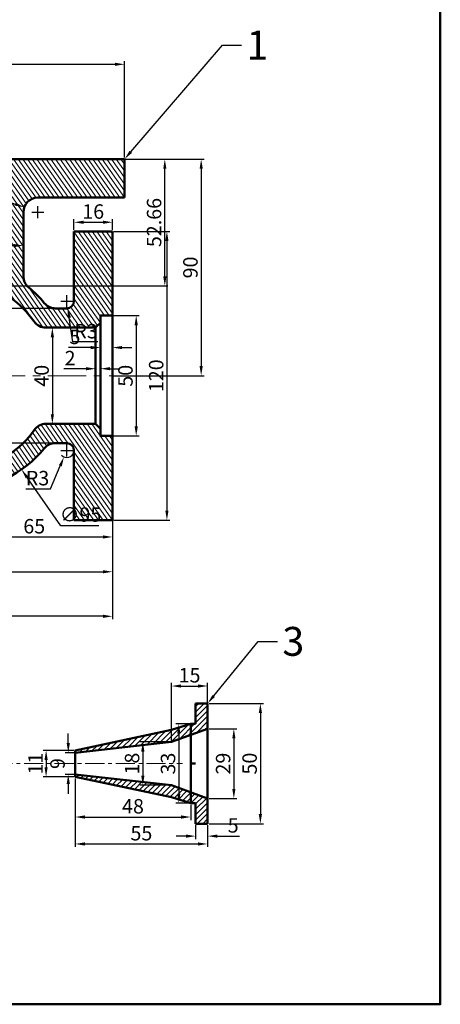
# Model space of a CAD drawing. Units: millimetres. Extents: x 39 to 520, y -165 to 464.
# Tile 3 of 4: x 345 to 520, y -165 to 244. Entities that reach past the tile are written whole.
import ezdxf
from ezdxf import colors
from ezdxf.entities.mleader import LeaderData, LeaderLine
from ezdxf.math import Vec2, Vec3

# ---------------------------------------------------------------- set-up
doc = ezdxf.new("R2010")
doc.units = ezdxf.units.MM
doc.header["$LTSCALE"] = 0.5
doc.linetypes.add('CENTER', pattern=[50.8, 31.75, -6.35, 6.35, -6.35])
for name, color, linetype, lineweight in [('M-CNTR', 1, 'CENTER', 18), ('M-DIMS', 2, 'Continuous', 25), ('M-HATC', 8, 'Continuous', 18), ('M-OUTL', 7, 'Continuous', 50), ('M-TEXT', 3, 'Continuous', 25), ('M-TTLB', 7, 'Continuous', 50)]:
    doc.layers.add(name, color=color, linetype=linetype, lineweight=lineweight)
doc.styles.get("Standard").update_dxf_attribs({"font": 'arial.ttf'})
doc.dimstyles.new('ISO-25', dxfattribs={"dimtxt": 6, "dimasz": 4, "dimexe": 1.25, "dimexo": 0.625, "dimtad": 1, "dimtoh": 1, "dimdec": 1, "dimtxsty": 'Standard', "dimcen": 2.5, "dimadec": 0, "dimazin": 0, "dimtfac": 1, "dimtdec": 1, "dimtofl": 0, "dimtmove": 0, "dimatfit": 3, "dimfxl": 1, "dimarcsym": 0})

# ---------------------------------------------------------------- blocks, each defined once
blk = doc.blocks.new('*D1')
at = {"layer": 'Defpoints', "color": 0, "ltscale": 0.5, "transparency": 16777216}
for p in [(388.62, 225.52), (248.62, 186.1), (388.62, 186.1)]:
    blk.add_point(p, dxfattribs=at)
at = {"layer": 'M-DIMS', "color": 0, "lineweight": -2, "ltscale": 0.5, "transparency": 16777216}
for p, q in [((248.62, 186.73), (248.62, 226.77)), ((252.62, 225.52), (384.62, 225.52)), ((388.62, 186.73), (388.62, 226.77))]:
    blk.add_line(p, q, dxfattribs=at)
at = {"layer": 'M-DIMS', "color": 0, "ltscale": 0.5, "transparency": 16777216}
for points in [[(252.62, 226.18), (252.62, 224.85), (248.62, 225.52)], [(384.62, 226.18), (384.62, 224.85), (388.62, 225.52)]]:
    blk.add_solid(points, dxfattribs=at)
at = {"layer": 'M-DIMS', "color": 0, "ltscale": 0.5, "transparency": 16777216, "insert": (318.62, 229.21), "char_height": 6, "attachment_point": 5}
blk.add_mtext('140', dxfattribs=at)
blk = doc.blocks.new('*D2')
at = {"layer": 'Defpoints', "color": 0, "ltscale": 0.5, "transparency": 16777216}
for p in [(290.62, 156.95), (346.62, 156.95), (346.62, 150.19)]:
    blk.add_point(p, dxfattribs=at)
at = {"layer": 'M-DIMS', "color": 0, "lineweight": -2, "ltscale": 0.5, "transparency": 16777216}
for p, q in [((290.62, 156.32), (290.62, 148.94)), ((346.62, 156.32), (346.62, 148.94)), ((294.62, 150.19), (342.62, 150.19))]:
    blk.add_line(p, q, dxfattribs=at)
at = {"layer": 'M-DIMS', "color": 0, "ltscale": 0.5, "transparency": 16777216}
for points in [[(294.62, 150.85), (294.62, 149.52), (290.62, 150.19)], [(342.62, 150.85), (342.62, 149.52), (346.62, 150.19)]]:
    blk.add_solid(points, dxfattribs=at)
at = {"layer": 'M-DIMS', "color": 0, "ltscale": 0.5, "transparency": 16777216, "insert": (318.62, 153.88), "char_height": 6, "attachment_point": 5}
blk.add_mtext('56', dxfattribs=at)
blk = doc.blocks.new('*D4')
at = {"layer": 'Defpoints', "color": 0, "ltscale": 0.5, "transparency": 16777216}
for p in [(383.62, 159.88), (367.62, 156.1), (383.62, 156.1)]:
    blk.add_point(p, dxfattribs=at)
at = {"layer": 'M-DIMS', "color": 0, "lineweight": -2, "ltscale": 0.5, "transparency": 16777216}
for p, q in [((367.62, 156.73), (367.62, 161.13)), ((371.62, 159.88), (379.62, 159.88)), ((383.62, 156.73), (383.62, 161.13))]:
    blk.add_line(p, q, dxfattribs=at)
at = {"layer": 'M-DIMS', "color": 0, "ltscale": 0.5, "transparency": 16777216}
for points in [[(371.62, 160.55), (371.62, 159.22), (367.62, 159.88)], [(379.62, 160.55), (379.62, 159.22), (383.62, 159.88)]]:
    blk.add_solid(points, dxfattribs=at)
at = {"layer": 'M-DIMS', "color": 0, "ltscale": 0.5, "transparency": 16777216, "insert": (375.62, 163.57), "char_height": 6, "attachment_point": 5}
blk.add_mtext('16', dxfattribs=at)
blk = doc.blocks.new('*D6')
at = {"layer": 'Defpoints', "color": 0, "ltscale": 0.5, "transparency": 16777216}
for p in [(388.62, 186.1), (383.62, 96.1), (420.47, 96.1)]:
    blk.add_point(p, dxfattribs=at)
at = {"layer": 'M-DIMS', "color": 0, "lineweight": -2, "ltscale": 0.5, "transparency": 16777216}
for p, q in [((389.25, 186.1), (421.72, 186.1)), ((420.47, 182.1), (420.47, 100.1)), ((384.25, 96.1), (421.72, 96.1))]:
    blk.add_line(p, q, dxfattribs=at)
at = {"layer": 'M-DIMS', "color": 0, "ltscale": 0.5, "transparency": 16777216}
for points in [[(419.81, 182.1), (421.14, 182.1), (420.47, 186.1)], [(419.81, 100.1), (421.14, 100.1), (420.47, 96.1)]]:
    blk.add_solid(points, dxfattribs=at)
at = {"layer": 'M-DIMS', "color": 0, "ltscale": 0.5, "transparency": 16777216, "insert": (416.78, 141.1), "char_height": 6, "attachment_point": 5, "rotation": 90}
blk.add_mtext('90', dxfattribs=at)
blk = doc.blocks.new('*D7')
at = {"layer": 'Defpoints', "color": 0, "ltscale": 0.5, "transparency": 16777216}
for p in [(383.62, 156.1), (383.62, 36.1), (406.24, 36.1)]:
    blk.add_point(p, dxfattribs=at)
at = {"layer": 'M-DIMS', "color": 0, "lineweight": -2, "ltscale": 0.5, "transparency": 16777216}
for p, q in [((384.25, 156.1), (407.49, 156.1)), ((406.24, 152.1), (406.24, 40.1)), ((384.25, 36.1), (407.49, 36.1))]:
    blk.add_line(p, q, dxfattribs=at)
at = {"layer": 'M-DIMS', "color": 0, "ltscale": 0.5, "transparency": 16777216}
for points in [[(405.57, 152.1), (406.9, 152.1), (406.24, 156.1)], [(405.57, 40.1), (406.9, 40.1), (406.24, 36.1)]]:
    blk.add_solid(points, dxfattribs=at)
at = {"layer": 'M-DIMS', "color": 0, "ltscale": 0.5, "transparency": 16777216, "insert": (402.55, 96.1), "char_height": 6, "attachment_point": 5, "rotation": 90}
blk.add_mtext('120', dxfattribs=at)
blk = doc.blocks.new('*D8')
at = {"layer": 'Defpoints', "color": 0, "ltscale": 0.5, "transparency": 16777216}
for p in [(383.62, 121.1), (383.62, 71.1), (393.48, 71.1)]:
    blk.add_point(p, dxfattribs=at)
at = {"layer": 'M-DIMS', "color": 0, "lineweight": -2, "ltscale": 0.5, "transparency": 16777216}
for p, q in [((384.25, 121.1), (394.73, 121.1)), ((393.48, 117.1), (393.48, 75.1)), ((384.25, 71.1), (394.73, 71.1))]:
    blk.add_line(p, q, dxfattribs=at)
at = {"layer": 'M-DIMS', "color": 0, "ltscale": 0.5, "transparency": 16777216}
for points in [[(392.81, 117.1), (394.15, 117.1), (393.48, 121.1)], [(392.81, 75.1), (394.15, 75.1), (393.48, 71.1)]]:
    blk.add_solid(points, dxfattribs=at)
at = {"layer": 'M-DIMS', "color": 0, "ltscale": 0.5, "transparency": 16777216, "insert": (389.79, 96.1), "char_height": 6, "attachment_point": 5, "rotation": 90}
blk.add_mtext('50', dxfattribs=at)
blk = doc.blocks.new('*D9')
at = {"layer": 'Defpoints', "color": 0, "ltscale": 0.5, "transparency": 16777216}
for p in [(378.62, 106.38), (383.62, 107.8), (383.62, 106.38)]:
    blk.add_point(p, dxfattribs=at)
at = {"layer": 'M-DIMS', "color": 0, "lineweight": -2, "ltscale": 0.5, "transparency": 16777216}
for p, q in [((374.62, 107.8), (365.39, 107.8)), ((378.62, 107.01), (378.62, 109.05)), ((383.62, 107.01), (383.62, 109.05)), ((387.62, 107.8), (391.62, 107.8))]:
    blk.add_line(p, q, dxfattribs=at)
at = {"layer": 'M-DIMS', "color": 0, "ltscale": 0.5, "transparency": 16777216}
for points in [[(374.62, 108.47), (374.62, 107.13), (378.62, 107.8)], [(387.62, 108.47), (387.62, 107.13), (383.62, 107.8)]]:
    blk.add_solid(points, dxfattribs=at)
at = {"layer": 'M-DIMS', "color": 0, "ltscale": 0.5, "transparency": 16777216, "insert": (368.01, 111.47), "char_height": 6, "attachment_point": 5}
blk.add_mtext('5', dxfattribs=at)
blk = doc.blocks.new('*D10')
at = {"layer": 'Defpoints', "color": 0, "ltscale": 0.5, "transparency": 16777216}
for p in [(376.62, 99.43), (378.62, 99.43), (378.62, 99.03)]:
    blk.add_point(p, dxfattribs=at)
at = {"layer": 'M-DIMS', "color": 0, "lineweight": -2, "ltscale": 0.5, "transparency": 16777216}
for p, q in [((372.62, 99.03), (363.4, 99.03)), ((376.62, 98.8), (376.62, 97.78)), ((378.62, 98.8), (378.62, 97.78)), ((382.62, 99.03), (386.62, 99.03))]:
    blk.add_line(p, q, dxfattribs=at)
at = {"layer": 'M-DIMS', "color": 0, "ltscale": 0.5, "transparency": 16777216}
for points in [[(372.62, 99.69), (372.62, 98.36), (376.62, 99.03)], [(382.62, 99.69), (382.62, 98.36), (378.62, 99.03)]]:
    blk.add_solid(points, dxfattribs=at)
at = {"layer": 'M-DIMS', "color": 0, "ltscale": 0.5, "transparency": 16777216, "insert": (366.01, 102.66), "char_height": 6, "attachment_point": 5}
blk.add_mtext('2', dxfattribs=at)
blk = doc.blocks.new('*D11')
at = {"layer": 'Defpoints', "color": 0, "ltscale": 0.5, "transparency": 16777216}
for p in [(318.62, 41.45), (383.62, 36.1), (383.62, 29.1)]:
    blk.add_point(p, dxfattribs=at)
at = {"layer": 'M-DIMS', "color": 0, "lineweight": -2, "ltscale": 0.5, "transparency": 16777216}
for p, q in [((318.62, 40.83), (318.62, 27.85)), ((383.62, 35.48), (383.62, 27.85)), ((322.62, 29.1), (379.62, 29.1))]:
    blk.add_line(p, q, dxfattribs=at)
at = {"layer": 'M-DIMS', "color": 0, "ltscale": 0.5, "transparency": 16777216}
for points in [[(322.62, 29.77), (322.62, 28.44), (318.62, 29.1)], [(379.62, 29.77), (379.62, 28.44), (383.62, 29.1)]]:
    blk.add_solid(points, dxfattribs=at)
at = {"layer": 'M-DIMS', "color": 0, "ltscale": 0.5, "transparency": 16777216, "insert": (351.12, 32.79), "char_height": 6, "attachment_point": 5}
blk.add_mtext('65', dxfattribs=at)
blk = doc.blocks.new('*D12')
at = {"layer": 'Defpoints', "color": 0, "ltscale": 0.5, "transparency": 16777216}
for p in [(283.62, 96.1), (383.62, 48.96), (383.62, 14.65)]:
    blk.add_point(p, dxfattribs=at)
at = {"layer": 'M-DIMS', "color": 0, "lineweight": -2, "ltscale": 0.5, "transparency": 16777216}
for p, q in [((283.62, 95.48), (283.62, 13.4)), ((383.62, 48.34), (383.62, 13.4)), ((287.62, 14.65), (379.62, 14.65))]:
    blk.add_line(p, q, dxfattribs=at)
at = {"layer": 'M-DIMS', "color": 0, "ltscale": 0.5, "transparency": 16777216}
for points in [[(287.62, 15.32), (287.62, 13.98), (283.62, 14.65)], [(379.62, 15.32), (379.62, 13.98), (383.62, 14.65)]]:
    blk.add_solid(points, dxfattribs=at)
at = {"layer": 'M-DIMS', "color": 0, "ltscale": 0.5, "transparency": 16777216, "insert": (333.62, 18.34), "char_height": 6, "attachment_point": 5}
blk.add_mtext('100', dxfattribs=at)
blk = doc.blocks.new('*D13')
at = {"layer": 'Defpoints', "color": 0, "ltscale": 0.5, "transparency": 16777216}
for p in [(153.62, 36.1), (383.62, 36.1), (153.62, -3.86)]:
    blk.add_point(p, dxfattribs=at)
at = {"layer": 'M-DIMS', "color": 0, "lineweight": -2, "ltscale": 0.5, "transparency": 16777216}
for p, q in [((153.62, 35.48), (153.62, -5.11)), ((383.62, 35.48), (383.62, -5.11)), ((379.62, -3.86), (157.62, -3.86))]:
    blk.add_line(p, q, dxfattribs=at)
at = {"layer": 'M-DIMS', "color": 0, "ltscale": 0.5, "transparency": 16777216}
for points in [[(157.62, -3.19), (157.62, -4.53), (153.62, -3.86)], [(379.62, -3.19), (379.62, -4.53), (383.62, -3.86)]]:
    blk.add_solid(points, dxfattribs=at)
at = {"layer": 'M-DIMS', "color": 0, "ltscale": 0.5, "transparency": 16777216, "insert": (268.62, -0.17), "char_height": 6, "attachment_point": 5}
blk.add_mtext('230', dxfattribs=at)
blk = doc.blocks.new('*D14')
at = {"layer": 'Defpoints', "color": 0, "ltscale": 0.5, "transparency": 16777216}
for p in [(359.93, 124.1), (340.68, 68.1), (362.28, 68.1)]:
    blk.add_point(p, dxfattribs=at)
at = {"layer": 'M-DIMS', "color": 0, "lineweight": -2, "ltscale": 0.5, "transparency": 16777216}
for p, q in [((359.3, 124.1), (339.43, 124.1)), ((340.68, 120.1), (340.68, 72.1)), ((361.65, 68.1), (339.43, 68.1))]:
    blk.add_line(p, q, dxfattribs=at)
at = {"layer": 'M-DIMS', "color": 0, "ltscale": 0.5, "transparency": 16777216}
for points in [[(340.02, 120.1), (341.35, 120.1), (340.68, 124.1)], [(340.02, 72.1), (341.35, 72.1), (340.68, 68.1)]]:
    blk.add_solid(points, dxfattribs=at)
at = {"layer": 'M-DIMS', "color": 0, "ltscale": 0.5, "transparency": 16777216, "insert": (337, 96.1), "char_height": 6, "attachment_point": 5, "rotation": 90}
blk.add_mtext('56', dxfattribs=at)
blk = doc.blocks.new('*D15')
at = {"layer": 'Defpoints', "color": 0, "ltscale": 0.5, "transparency": 16777216}
for p in [(361.76, 116.1), (358.64, 76.1), (361.76, 76.1)]:
    blk.add_point(p, dxfattribs=at)
at = {"layer": 'M-DIMS', "color": 0, "lineweight": -2, "ltscale": 0.5, "transparency": 16777216}
for p, q in [((361.13, 116.1), (357.39, 116.1)), ((358.64, 112.1), (358.64, 80.1)), ((361.13, 76.1), (357.39, 76.1))]:
    blk.add_line(p, q, dxfattribs=at)
at = {"layer": 'M-DIMS', "color": 0, "ltscale": 0.5, "transparency": 16777216}
for points in [[(357.98, 112.1), (359.31, 112.1), (358.64, 116.1)], [(357.98, 80.1), (359.31, 80.1), (358.64, 76.1)]]:
    blk.add_solid(points, dxfattribs=at)
at = {"layer": 'M-DIMS', "color": 0, "ltscale": 0.5, "transparency": 16777216, "insert": (354.95, 96.1), "char_height": 6, "attachment_point": 5, "rotation": 90}
blk.add_mtext('40', dxfattribs=at)
blk = doc.blocks.new('*D30')
at = {"layer": 'Defpoints', "color": 0, "ltscale": 0.5, "transparency": 16777216}
for p in [(363.47, 62.33), (364.62, 65.1)]:
    blk.add_point(p, dxfattribs=at)
at = {"layer": 'M-DIMS', "color": 0, "lineweight": -2, "ltscale": 0.5, "transparency": 16777216}
for p, q in [((364.62, 62.6), (364.62, 67.6)), ((362.12, 65.1), (367.12, 65.1)), ((357.94, 49.09), (361.93, 58.64)), ((347.64, 49.09), (357.94, 49.09))]:
    blk.add_line(p, q, dxfattribs=at)
blk.add_arc((364.62, 65.1), 3, 223.4691, 348.0634, dxfattribs=at)
at = {"layer": 'M-DIMS', "color": 0, "ltscale": 0.5, "transparency": 16777216}
blk.add_solid([(361.31, 58.9), (362.54, 58.39), (363.47, 62.33)], dxfattribs=at)
at = {"layer": 'M-DIMS', "color": 0, "ltscale": 0.5, "transparency": 16777216, "insert": (352.48, 52.78), "char_height": 6, "attachment_point": 5}
blk.add_mtext('R3', dxfattribs=at)
blk = doc.blocks.new('*D48')
at = {"layer": 'Defpoints', "color": 0, "ltscale": 0.5, "transparency": 16777216}
for p in [(423.14, -32.82), (408.14, -56.06), (423.14, -56.06)]:
    blk.add_point(p, dxfattribs=at)
at = {"layer": 'M-DIMS', "color": 0, "lineweight": -2, "ltscale": 0.5, "transparency": 16777216}
for p, q in [((408.14, -55.44), (408.14, -31.57)), ((423.14, -55.44), (423.14, -31.57)), ((412.14, -32.82), (419.14, -32.82))]:
    blk.add_line(p, q, dxfattribs=at)
at = {"layer": 'M-DIMS', "color": 0, "ltscale": 0.5, "transparency": 16777216}
for points in [[(412.14, -32.16), (412.14, -33.49), (408.14, -32.82)], [(419.14, -32.16), (419.14, -33.49), (423.14, -32.82)]]:
    blk.add_solid(points, dxfattribs=at)
at = {"layer": 'M-DIMS', "color": 0, "ltscale": 0.5, "transparency": 16777216, "insert": (415.64, -29.14), "char_height": 6, "attachment_point": 5}
blk.add_mtext('15', dxfattribs=at)
blk = doc.blocks.new('*D49')
at = {"layer": 'Defpoints', "color": 0, "ltscale": 0.5, "transparency": 16777216}
for p in [(423.14, -50.56), (423.14, -79.56), (434.05, -79.56)]:
    blk.add_point(p, dxfattribs=at)
at = {"layer": 'M-DIMS', "color": 0, "lineweight": -2, "ltscale": 0.5, "transparency": 16777216}
for p, q in [((423.77, -50.56), (435.3, -50.56)), ((434.05, -54.56), (434.05, -75.56)), ((423.77, -79.56), (435.3, -79.56))]:
    blk.add_line(p, q, dxfattribs=at)
at = {"layer": 'M-DIMS', "color": 0, "ltscale": 0.5, "transparency": 16777216}
for points in [[(433.39, -54.56), (434.72, -54.56), (434.05, -50.56)], [(433.39, -75.56), (434.72, -75.56), (434.05, -79.56)]]:
    blk.add_solid(points, dxfattribs=at)
at = {"layer": 'M-DIMS', "color": 0, "ltscale": 0.5, "transparency": 16777216, "insert": (430.37, -65.06), "char_height": 6, "attachment_point": 5, "rotation": 90}
blk.add_mtext('29', dxfattribs=at)
blk = doc.blocks.new('*D50')
at = {"layer": 'Defpoints', "color": 0, "ltscale": 0.5, "transparency": 16777216}
for p in [(423.14, -40.06), (423.14, -90.06), (445.07, -90.06)]:
    blk.add_point(p, dxfattribs=at)
at = {"layer": 'M-DIMS', "color": 0, "lineweight": -2, "ltscale": 0.5, "transparency": 16777216}
for p, q in [((423.77, -40.06), (446.32, -40.06)), ((445.07, -44.06), (445.07, -86.06)), ((423.77, -90.06), (446.32, -90.06))]:
    blk.add_line(p, q, dxfattribs=at)
at = {"layer": 'M-DIMS', "color": 0, "ltscale": 0.5, "transparency": 16777216}
for points in [[(444.4, -44.06), (445.74, -44.06), (445.07, -40.06)], [(444.4, -86.06), (445.74, -86.06), (445.07, -90.06)]]:
    blk.add_solid(points, dxfattribs=at)
at = {"layer": 'M-DIMS', "color": 0, "ltscale": 0.5, "transparency": 16777216, "insert": (441.38, -65.06), "char_height": 6, "attachment_point": 5, "rotation": 90}
blk.add_mtext('50', dxfattribs=at)
blk = doc.blocks.new('*D51')
at = {"layer": 'Defpoints', "color": 0, "ltscale": 0.5, "transparency": 16777216}
for p in [(368.14, -70.56), (423.14, -90.06), (423.14, -98.46)]:
    blk.add_point(p, dxfattribs=at)
at = {"layer": 'M-DIMS', "color": 0, "lineweight": -2, "ltscale": 0.5, "transparency": 16777216}
for p, q in [((368.14, -71.19), (368.14, -99.71)), ((423.14, -90.69), (423.14, -99.71)), ((372.14, -98.46), (419.14, -98.46))]:
    blk.add_line(p, q, dxfattribs=at)
at = {"layer": 'M-DIMS', "color": 0, "ltscale": 0.5, "transparency": 16777216}
for points in [[(372.14, -97.79), (372.14, -99.12), (368.14, -98.46)], [(419.14, -97.79), (419.14, -99.12), (423.14, -98.46)]]:
    blk.add_solid(points, dxfattribs=at)
at = {"layer": 'M-DIMS', "color": 0, "ltscale": 0.5, "transparency": 16777216, "insert": (395.64, -94.78), "char_height": 6, "attachment_point": 5}
blk.add_mtext('55', dxfattribs=at)
blk = doc.blocks.new('*D52')
at = {"layer": 'Defpoints', "color": 0, "ltscale": 0.5, "transparency": 16777216}
for p in [(368.14, -76.99), (416.14, -81.56), (416.14, -87.26)]:
    blk.add_point(p, dxfattribs=at)
at = {"layer": 'M-DIMS', "color": 0, "lineweight": -2, "ltscale": 0.5, "transparency": 16777216}
for p, q in [((368.14, -77.62), (368.14, -88.51)), ((416.14, -82.19), (416.14, -88.51)), ((372.14, -87.26), (412.14, -87.26))]:
    blk.add_line(p, q, dxfattribs=at)
at = {"layer": 'M-DIMS', "color": 0, "ltscale": 0.5, "transparency": 16777216}
for points in [[(372.14, -86.59), (372.14, -87.93), (368.14, -87.26)], [(412.14, -86.59), (412.14, -87.93), (416.14, -87.26)]]:
    blk.add_solid(points, dxfattribs=at)
at = {"layer": 'M-DIMS', "color": 0, "ltscale": 0.5, "transparency": 16777216, "insert": (392.14, -83.57), "char_height": 6, "attachment_point": 5}
blk.add_mtext('48', dxfattribs=at)
blk = doc.blocks.new('*D53')
at = {"layer": 'Defpoints', "color": 0, "ltscale": 0.5, "transparency": 16777216}
for p in [(368.14, -60.56), (365.25, -69.56), (368.14, -69.56)]:
    blk.add_point(p, dxfattribs=at)
at = {"layer": 'M-DIMS', "color": 0, "lineweight": -2, "ltscale": 0.5, "transparency": 16777216}
for p, q in [((365.25, -56.56), (365.25, -52.56)), ((367.52, -60.56), (364, -60.56)), ((367.52, -69.56), (364, -69.56)), ((365.25, -73.56), (365.25, -77.56))]:
    blk.add_line(p, q, dxfattribs=at)
at = {"layer": 'M-DIMS', "color": 0, "ltscale": 0.5, "transparency": 16777216}
for points in [[(364.59, -56.56), (365.92, -56.56), (365.25, -60.56)], [(364.59, -73.56), (365.92, -73.56), (365.25, -69.56)]]:
    blk.add_solid(points, dxfattribs=at)
at = {"layer": 'M-DIMS', "color": 0, "ltscale": 0.5, "transparency": 16777216, "insert": (361.56, -65.06), "char_height": 6, "attachment_point": 5, "rotation": 90}
blk.add_mtext('9', dxfattribs=at)
blk = doc.blocks.new('*D54')
at = {"layer": 'Defpoints', "color": 0, "ltscale": 0.5, "transparency": 16777216}
for p in [(368.14, -59.56), (356.04, -70.56), (368.14, -70.56)]:
    blk.add_point(p, dxfattribs=at)
at = {"layer": 'M-DIMS', "color": 0, "lineweight": -2, "ltscale": 0.5, "transparency": 16777216}
for p, q in [((367.52, -59.56), (354.79, -59.56)), ((356.04, -63.56), (356.04, -66.56)), ((367.52, -70.56), (354.79, -70.56))]:
    blk.add_line(p, q, dxfattribs=at)
at = {"layer": 'M-DIMS', "color": 0, "ltscale": 0.5, "transparency": 16777216}
for points in [[(355.37, -63.56), (356.71, -63.56), (356.04, -59.56)], [(355.37, -66.56), (356.71, -66.56), (356.04, -70.56)]]:
    blk.add_solid(points, dxfattribs=at)
at = {"layer": 'M-DIMS', "color": 0, "ltscale": 0.5, "transparency": 16777216, "insert": (352.4, -65.06), "char_height": 6, "attachment_point": 5, "rotation": 90}
blk.add_mtext('11', dxfattribs=at)
blk = doc.blocks.new('*D55')
at = {"layer": 'Defpoints', "color": 0, "ltscale": 0.5, "transparency": 16777216}
for p in [(418.14, -48.56), (411.17, -81.56), (418.14, -81.56)]:
    blk.add_point(p, dxfattribs=at)
at = {"layer": 'M-DIMS', "color": 0, "lineweight": -2, "ltscale": 0.5, "transparency": 16777216}
for p, q in [((417.52, -48.56), (409.92, -48.56)), ((411.17, -52.56), (411.17, -77.56)), ((417.52, -81.56), (409.92, -81.56))]:
    blk.add_line(p, q, dxfattribs=at)
at = {"layer": 'M-DIMS', "color": 0, "ltscale": 0.5, "transparency": 16777216}
for points in [[(410.51, -52.56), (411.84, -52.56), (411.17, -48.56)], [(410.51, -77.56), (411.84, -77.56), (411.17, -81.56)]]:
    blk.add_solid(points, dxfattribs=at)
at = {"layer": 'M-DIMS', "color": 0, "ltscale": 0.5, "transparency": 16777216, "insert": (407.48, -65.06), "char_height": 6, "attachment_point": 5, "rotation": 90}
blk.add_mtext('33', dxfattribs=at)
blk = doc.blocks.new('*D56')
at = {"layer": 'Defpoints', "color": 0, "ltscale": 0.5, "transparency": 16777216}
for p in [(408.14, -56.06), (396.23, -74.06), (408.14, -74.06)]:
    blk.add_point(p, dxfattribs=at)
at = {"layer": 'M-DIMS', "color": 0, "lineweight": -2, "ltscale": 0.5, "transparency": 16777216}
for p, q in [((407.52, -56.06), (394.98, -56.06)), ((396.23, -60.06), (396.23, -70.06)), ((407.52, -74.06), (394.98, -74.06))]:
    blk.add_line(p, q, dxfattribs=at)
at = {"layer": 'M-DIMS', "color": 0, "ltscale": 0.5, "transparency": 16777216}
for points in [[(395.56, -60.06), (396.9, -60.06), (396.23, -56.06)], [(395.56, -70.06), (396.9, -70.06), (396.23, -74.06)]]:
    blk.add_solid(points, dxfattribs=at)
at = {"layer": 'M-DIMS', "color": 0, "ltscale": 0.5, "transparency": 16777216, "insert": (392.54, -65.06), "char_height": 6, "attachment_point": 5, "rotation": 90}
blk.add_mtext('18', dxfattribs=at)
blk = doc.blocks.new('*D57')
at = {"layer": 'Defpoints', "color": 0, "ltscale": 0.5, "transparency": 16777216}
for p in [(418.14, -90.06), (423.14, -90.06), (423.14, -95.2)]:
    blk.add_point(p, dxfattribs=at)
at = {"layer": 'M-DIMS', "color": 0, "lineweight": -2, "ltscale": 0.5, "transparency": 16777216}
for p, q in [((418.14, -90.69), (418.14, -96.45)), ((423.14, -90.69), (423.14, -96.45)), ((414.14, -95.2), (410.14, -95.2)), ((427.14, -95.2), (436.37, -95.2))]:
    blk.add_line(p, q, dxfattribs=at)
at = {"layer": 'M-DIMS', "color": 0, "ltscale": 0.5, "transparency": 16777216}
for points in [[(414.14, -94.53), (414.14, -95.86), (418.14, -95.2)], [(427.14, -94.53), (427.14, -95.86), (423.14, -95.2)]]:
    blk.add_solid(points, dxfattribs=at)
at = {"layer": 'M-DIMS', "color": 0, "ltscale": 0.5, "transparency": 16777216, "insert": (433.76, -91.52), "char_height": 6, "attachment_point": 5}
blk.add_mtext('5', dxfattribs=at)
blk = doc.blocks.new('*D58')
at = {"layer": 'Defpoints', "color": 0, "ltscale": 0.5, "transparency": 16777216}
for p in [(338.62, 186.1), (405.37, 186.1), (338.62, 133.44)]:
    blk.add_point(p, dxfattribs=at)
at = {"layer": 'M-DIMS', "color": 0, "lineweight": -2, "ltscale": 0.5, "transparency": 16777216}
for p, q in [((339.25, 186.1), (406.62, 186.1)), ((405.37, 137.44), (405.37, 182.1)), ((339.25, 133.44), (406.62, 133.44))]:
    blk.add_line(p, q, dxfattribs=at)
at = {"layer": 'M-DIMS', "color": 0, "ltscale": 0.5, "transparency": 16777216}
for points in [[(404.71, 182.1), (406.04, 182.1), (405.37, 186.1)], [(404.71, 137.44), (406.04, 137.44), (405.37, 133.44)]]:
    blk.add_solid(points, dxfattribs=at)
at = {"layer": 'M-DIMS', "color": 0, "ltscale": 0.5, "transparency": 16777216, "insert": (401.68, 159.77), "char_height": 6, "attachment_point": 5, "rotation": 90}
blk.add_mtext('52.66', dxfattribs=at)
blk = doc.blocks.new('*D62')
at = {"layer": 'Defpoints', "color": 0, "ltscale": 0.5, "transparency": 16777216}
for p in [(364.62, 127.1), (365.07, 124.14)]:
    blk.add_point(p, dxfattribs=at)
at = {"layer": 'M-DIMS', "color": 0, "lineweight": -2, "ltscale": 0.5, "transparency": 16777216}
for p, q in [((362.12, 127.1), (367.12, 127.1)), ((364.62, 124.6), (364.62, 129.6)), ((367.18, 110.16), (365.67, 120.18)), ((377.48, 110.16), (367.18, 110.16))]:
    blk.add_line(p, q, dxfattribs=at)
at = {"layer": 'M-DIMS', "color": 0, "ltscale": 0.5, "transparency": 16777216}
blk.add_solid([(366.33, 120.28), (365.01, 120.08), (365.07, 124.14)], dxfattribs=at)
at = {"layer": 'M-DIMS', "color": 0, "ltscale": 0.5, "transparency": 16777216, "insert": (372.64, 113.85), "char_height": 6, "attachment_point": 5}
blk.add_mtext('R3', dxfattribs=at)
blk = doc.blocks.new('*D64')
at = {"layer": 'Defpoints', "color": 0, "ltscale": 0.5, "transparency": 16777216}
for p in [(291.42, 135.04), (345.83, 57.16)]:
    blk.add_point(p, dxfattribs=at)
at = {"layer": 'M-DIMS', "color": 0, "lineweight": -2, "ltscale": 0.5, "transparency": 16777216}
for p, q in [((318.62, 93.6), (318.62, 98.6)), ((316.12, 96.1), (321.12, 96.1)), ((362.15, 33.8), (348.12, 53.88)), ((377.94, 33.8), (362.15, 33.8))]:
    blk.add_line(p, q, dxfattribs=at)
at = {"layer": 'M-DIMS', "color": 0, "ltscale": 0.5, "transparency": 16777216}
blk.add_solid([(348.66, 54.27), (347.57, 53.5), (345.83, 57.16)], dxfattribs=at)
at = {"layer": 'M-DIMS', "color": 0, "ltscale": 0.5, "transparency": 16777216, "insert": (370.36, 37.66), "char_height": 6, "attachment_point": 5}
blk.add_mtext('∅95', dxfattribs=at)
blk = doc.blocks.new('*D69')
at = {"layer": 'Defpoints', "color": 0, "ltscale": 0.5, "transparency": 16777216}
for p in [(346.97, 166.1), (352.62, 164.1)]:
    blk.add_point(p, dxfattribs=at)
at = {"layer": 'M-DIMS', "color": 0, "lineweight": -2, "ltscale": 0.5, "transparency": 16777216}
for p, q in [((300.5, 168.77), (339.42, 168.77)), ((339.42, 168.77), (343.19, 167.44)), ((350.12, 164.1), (355.12, 164.1)), ((352.62, 161.6), (352.62, 166.6))]:
    blk.add_line(p, q, dxfattribs=at)
at = {"layer": 'M-DIMS', "color": 0, "ltscale": 0.5, "transparency": 16777216}
blk.add_solid([(343.42, 168.06), (342.97, 166.81), (346.97, 166.1)], dxfattribs=at)
at = {"layer": 'M-DIMS', "color": 0, "ltscale": 0.5, "transparency": 16777216, "insert": (319.65, 172.46), "char_height": 6, "attachment_point": 5}
blk.add_mtext('12X R6.00', dxfattribs=at)

msp = doc.modelspace()

# ---------------------------------------------------------------- hatches: boundary and pattern name
at = {"layer": 'M-HATC', "ltscale": 0.5}
h = msp.add_hatch(dxfattribs=at)
h.set_pattern_fill('ANSI31', color=256, scale=0.5, angle=80)
h.paths.add_polyline_path([(296.0512, 128.5189, 0.24539268), (298.6226, 133.4428), (298.6226, 186.1031), (248.6226, 186.1031), (248.6226, 170.1031), (284.6226, 170.1031, -0.41421356), (290.6226, 164.1031), (290.6226, 137.4099, -0.22417658), (288.4357, 132.7774, 0.04839978), (281.9483, 126.29, -0.17668241), (278.4054, 124.2029), (169.6226, 128.6031), (169.6226, 166.1031), (153.6226, 166.1031), (153.6226, 124.1031), (158.6226, 124.1031), (158.6226, 120.1031, 0.17132661), (164.3106, 118.1031), (272.6226, 118.1031, -0.41421356), (275.6226, 115.1031), (275.6226, 114.6031), (283.7227, 114.6031, -0.11934263)])
h.paths.add_polyline_path([(283.7227, 77.6031), (275.6226, 77.6031), (275.6226, 77.1031, -0.41421356), (272.6226, 74.1031), (164.2881, 74.1031, 0.17068716), (158.6226, 72.1031), (158.6226, 68.1031), (153.6226, 68.1031), (153.6226, 26.1031), (169.6226, 26.1031), (169.6226, 63.6031), (276.6027, 67.9304, -0.16745848), (283.458, 64.1703, 0.21145125), (318.6226, 48.6031), (318.6226, 56.6031, -0.27766509)])
h.paths.add_polyline_path([(355.2968, 65.9162, -0.22417658), (359.9294, 68.1031), (364.6226, 68.1031, -0.41421356), (367.6226, 65.1031), (367.6226, 36.1031), (383.6226, 36.1031), (383.6226, 71.1031), (378.6226, 71.1031), (378.6226, 74.1031), (376.6226, 76.1031), (355.9622, 76.1031, 0.24539268), (351.0383, 73.5317, -0.24539268), (318.6226, 56.6031), (318.6226, 48.6031, 0.22417658)])
h.paths.add_polyline_path([(383.6226, 156.1031), (367.6226, 156.1031), (367.6226, 127.1031, -0.41421356), (364.6226, 124.1031), (359.9294, 124.1031, -0.22417658), (355.2968, 126.29, 0.04839978), (348.8095, 132.7774, -0.22417658), (346.6226, 137.4099), (346.6226, 164.1031, -0.41421356), (352.6226, 170.1031), (388.6226, 170.1031), (388.6226, 186.1031), (338.6226, 186.1031), (338.6226, 133.4428, 0.24539268), (341.194, 128.5189, -0.08880867), (351.0383, 118.6745, 0.24539268), (355.9622, 116.1031), (376.6226, 116.1031), (378.6226, 118.1031), (378.6226, 121.1031), (383.6226, 121.1031)])
h = msp.add_hatch(dxfattribs=at)
h.set_pattern_fill('ANSI31', color=256, scale=0.5)
h.set_pattern_definition([(45, (-121.1096, 1323.1625), (-1.122532, 1.122532), [])])
h.paths.add_polyline_path([(423.141, -50.5616), (423.141, -40.0616), (418.141, -40.0616), (418.141, -48.5616), (416.141, -48.5616), (408.141, -51.0616), (368.141, -59.5616), (368.141, -60.5616), (408.141, -56.0616)])
h.paths.add_polyline_path([(368.141, -69.5616), (368.141, -70.5616), (408.141, -79.0616), (416.141, -81.5616), (418.141, -81.5616), (418.141, -90.0616), (423.141, -90.0616), (423.141, -79.5616), (408.141, -74.0616)])

# ---------------------------------------------------------------- linework, layer by layer
at = {"layer": 'M-CNTR'}
msp.add_line((153.6226, 96.1031), (383.6226, 96.1031), dxfattribs=at)
at = {"layer": 'M-CNTR', "ltscale": 0.5}
msp.add_line((143.7018, -65.0616), (412.7093, -65.0616), dxfattribs=at)
at = {"layer": 'M-OUTL'}
for p, q in [((388.6226, 186.1031), (248.6226, 186.1031)), ((388.6226, 170.1031), (388.6226, 186.1031)), ((352.6226, 170.1031), (388.6226, 170.1031)), ((346.6226, 137.4099), (346.6226, 164.1031)), ((383.6226, 156.1031), (367.6226, 156.1031)), ((367.6226, 156.1031), (367.6226, 127.1031)), ((383.6226, 96.1031), (383.6226, 156.1031)), ((364.6226, 124.1031), (359.9294, 124.1031))]:
    msp.add_line(p, q, dxfattribs=at)
at = {"layer": 'M-OUTL', "ltscale": 0.5}
for p, q in [((423.141, -40.0616), (418.141, -40.0616)), ((418.141, -40.0616), (418.141, -48.5616)), ((423.141, -65.0616), (423.141, -40.0616)), ((408.141, -51.0616), (416.141, -48.5616)), ((416.141, -48.5616), (418.141, -48.5616)), ((416.141, -48.5616), (416.141, -81.5616)), ((368.141, -59.5616), (408.141, -51.0616)), ((423.141, -50.5616), (408.141, -56.0616)), ((408.141, -56.0616), (368.141, -60.5616)), ((368.141, -70.5616), (368.141, -59.5616)), ((423.141, -65.0616), (423.141, -59.2443)), ((416.141, -65.0616), (418.141, -65.0616)), ((423.141, -90.0616), (423.141, -65.0616)), ((368.141, -69.5616), (408.141, -74.0616)), ((368.141, -70.5616), (408.141, -79.0616)), ((408.141, -74.0616), (423.141, -79.5616)), ((408.141, -79.0616), (416.141, -81.5616)), ((416.141, -81.5616), (418.141, -81.5616)), ((418.141, -81.5616), (418.141, -90.0616)), ((418.141, -90.0616), (423.141, -90.0616))]:
    msp.add_line(p, q, dxfattribs=at)
at = {"layer": 'M-OUTL'}
for points in [[(338.6226, 186.1031), (338.6226, 133.4428, 0.24539268), (341.194, 128.5189, -0.08880867), (351.0383, 118.6745, 0.24539268), (355.9622, 116.1031), (376.6226, 116.1031)], [(153.6226, 166.1031), (153.6226, 26.1031), (169.6226, 26.1031), (169.6226, 63.6031), (276.6027, 67.9304, -0.16745848), (283.458, 64.1703, 0.4573052), (355.2968, 65.9162, -0.22417658), (359.9294, 68.1031), (364.6226, 68.1031, -0.41421356), (367.6226, 65.1031), (367.6226, 36.1031), (383.6226, 36.1031), (383.6226, 96.1031)], [(283.6226, 77.7933, 0.5630935), (351.0383, 73.5317, -0.24539268), (355.9622, 76.1031), (376.6226, 76.1031)]]:
    msp.add_lwpolyline(points, format="xyb", dxfattribs=at)
for points in [[(378.6226, 118.1031), (376.6226, 116.1031), (376.6226, 76.1031), (378.6226, 74.1031), (378.6226, 121.1031), (383.6226, 121.1031)], [(378.6226, 74.1031), (378.6226, 71.1031), (383.6226, 71.1031)]]:
    msp.add_lwpolyline(points, dxfattribs=at)
for centre, radius, start, end in [((352.6226, 164.1031), 6, 90, 180), ((352.6226, 137.4099), 6, 180, 230.541881), ((318.6226, 96.1031), 47.5, 39.458119, 50.541881), ((364.6226, 127.1031), 3, 270, 0), ((359.9294, 130.1031), 6, 219.458119, 270)]:
    msp.add_arc(centre, radius, start, end, dxfattribs=at)
at = {"layer": 'M-TTLB', "ltscale": 0.5}
msp.add_lwpolyline([(39.27, 463.9335), (519.8288, 463.9335), (519.8288, -165.0878), (39.27, -165.0878)], close=True, dxfattribs=at)

# ---------------------------------------------------------------- dimensions: what is measured, and where the dimension line sits
at = {"layer": 'M-DIMS', "ltscale": 0.5}
for base, p1, p2, picture, middle in [((388.6226, 225.517), (248.6226, 186.1031), (388.6226, 186.1031), '*D1', (318.6226, 229.2054)), ((383.6226, 159.8838), (367.6226, 156.1031), (383.6226, 156.1031), '*D4', (375.6226, 163.5722)), ((346.6226, 150.1873), (290.6226, 156.9452), (346.6226, 156.9452), '*D2', (318.6226, 153.8757)), ((383.6226, 14.6514), (283.6226, 96.1031), (383.6226, 48.9607), '*D12', (333.6226, 18.3398)), ((383.6226, 29.1036), (318.6226, 41.4507), (383.6226, 36.1031), '*D11', (351.1226, 32.7921)), ((153.6226, -3.8615), (383.6226, 36.1031), (153.6226, 36.1031), '*D13', (268.6226, -0.171)), ((423.141, -32.8245), (408.141, -56.0616), (423.141, -56.0616), '*D48', (415.641, -29.1361)), ((423.141, -98.4583), (368.141, -70.5616), (423.141, -90.0616), '*D51', (395.641, -94.7821)), ((416.141, -87.2608), (368.141, -76.9922), (416.141, -81.5616), '*D52', (392.141, -83.5724)), ((423.141, -95.1974), (418.141, -90.0616), (423.141, -90.0616), '*D57', (433.7551, -91.5213))]:
    dim = msp.add_linear_dim(base=base, p1=p1, p2=p2, dimstyle='ISO-25', override={"dimclrd": 0, "dimclre": 0, "dimclrt": 0}, dxfattribs=at)
    dim.commit()
    dim.dimension.update_dxf_attribs({"geometry": picture, "text_midpoint": middle})
for base, p1, p2, override, picture, middle in [((405.3726, 186.1031), (338.6226, 133.4428), (338.6226, 186.1031), {"dimdec": 2, "dimlfac": 1, "dimrnd": 0, "dimzin": 0, "dimdsep": 46, "dimlunit": 2}, '*D58', (401.6842, 159.7729)), ((420.4729, 96.1031), (388.6226, 186.1031), (383.6226, 96.1031), {"dimclrd": 0, "dimclre": 0, "dimclrt": 0}, '*D6', (416.7845, 141.1031)), ((406.2372, 36.1031), (383.6226, 156.1031), (383.6226, 36.1031), {"dimclrd": 0, "dimclre": 0, "dimclrt": 0}, '*D7', (402.5488, 96.1031)), ((340.6837, 68.1031), (359.9294, 124.1031), (362.276, 68.1031), {"dimclrd": 0, "dimclre": 0, "dimclrt": 0}, '*D14', (336.9953, 96.1031)), ((393.4798, 71.1031), (383.6226, 121.1031), (383.6226, 71.1031), {"dimclrd": 0, "dimclre": 0, "dimclrt": 0}, '*D8', (389.7913, 96.1031)), ((358.642, 76.1031), (361.756, 116.1031), (361.756, 76.1031), {"dimclrd": 0, "dimclre": 0, "dimclrt": 0}, '*D15', (354.9535, 96.1031)), ((445.0699, -90.0616), (423.141, -40.0616), (423.141, -90.0616), {"dimclrd": 0, "dimclre": 0, "dimclrt": 0}, '*D50', (441.3815, -65.0616)), ((411.1722, -81.5616), (418.141, -48.5616), (418.141, -81.5616), {"dimclrd": 0, "dimclre": 0, "dimclrt": 0}, '*D55', (407.4818, -65.0616)), ((365.2532, -69.5616), (368.141, -60.5616), (368.141, -69.5616), {"dimclrd": 0, "dimclre": 0, "dimclrt": 0}, '*D53', (361.5648, -65.0616)), ((434.0543, -79.5616), (423.141, -50.5616), (423.141, -79.5616), {"dimclrd": 0, "dimclre": 0, "dimclrt": 0}, '*D49', (430.3659, -65.0616)), ((396.2291, -74.0616), (408.141, -56.0616), (408.141, -74.0616), {"dimclrd": 0, "dimclre": 0, "dimclrt": 0}, '*D56', (392.5407, -65.0616)), ((356.0386, -70.5616), (368.141, -59.5616), (368.141, -70.5616), {"dimclrd": 0, "dimclre": 0, "dimclrt": 0}, '*D54', (352.4014, -65.0616))]:
    dim = msp.add_linear_dim(base=base, p1=p1, p2=p2, angle=90, dimstyle='ISO-25', override=override, dxfattribs=at)
    dim.commit()
    dim.dimension.update_dxf_attribs({"geometry": picture, "text_midpoint": middle})
dim = msp.add_radius_dim(center=(352.6226, 164.1031), mpoint=(346.9657, 166.1031), text='12X <>', dimstyle='ISO-25', override={"dimdec": 2, "dimlfac": 1, "dimrnd": 0, "dimzin": 0, "dimdsep": 46, "dimlunit": 2}, dxfattribs=at)
dim.commit()
dim.dimension.update_dxf_attribs({"geometry": '*D69', "text_midpoint": (319.6502, 172.4581)})
dim = msp.add_diameter_dim_2p(p1=(291.4199, 135.0424), p2=(345.8252, 57.1639), dimstyle='ISO-25', override={"dimdec": 0, "dimlfac": 1, "dimrnd": 0, "dimzin": 0, "dimdsep": 46, "dimlunit": 2}, dxfattribs=at)
dim.commit()
dim.dimension.update_dxf_attribs({"geometry": '*D64', "text_midpoint": (370.3557, 33.8003), "dimtype": 163})
dim = msp.add_radius_dim(center=(364.6226, 127.1031), mpoint=(365.0699, 124.1366), dimstyle='ISO-25', override={"dimdec": 0, "dimlfac": 1, "dimrnd": 0, "dimzin": 0, "dimdsep": 46, "dimlunit": 2}, dxfattribs=at)
dim.commit()
dim.dimension.update_dxf_attribs({"geometry": '*D62', "text_midpoint": (372.6393, 113.8541)})
for base, p1, p2, picture, middle in [((383.6226, 107.7987), (378.6226, 106.3822), (383.6226, 106.3822), '*D9', (368.0085, 107.7987)), ((378.6226, 99.0276), (376.6226, 99.4291), (378.6226, 99.4291), '*D10', (366.0106, 99.0276))]:
    dim = msp.add_linear_dim(base=base, p1=p1, p2=p2, dimstyle='ISO-25', override={"dimclrd": 0, "dimclre": 0, "dimclrt": 0}, dxfattribs=at)
    dim.commit()
    dim.dimension.update_dxf_attribs({"geometry": picture, "text_midpoint": middle, "dimtype": 160})
dim = msp.add_radius_dim(center=(364.6226, 65.1031), mpoint=(363.4669, 62.3346), dimstyle='ISO-25', override={"dimclrd": 0, "dimclre": 0, "dimclrt": 0}, dxfattribs=at)
dim.commit()
dim.dimension.update_dxf_attribs({"geometry": '*D30', "text_midpoint": (352.4772, 49.0944), "dimtype": 164})

# ---------------------------------------------------------------- leaders
at = {"layer": 'M-TEXT', "ltscale": 0.5}
ml = msp.add_multileader_mtext('Standard', dxfattribs=at)
ml.set_content('1', color=256)
ml.set_leader_properties()
ml.build(insert=Vec2(0, 0))
ctx = ml.context
ctx.base_point, ctx.char_height, ctx.plane_origin = Vec3(437.27, 233.5108), 12, Vec3(388.6226, 186.1031)
notes = []
notes.append((ctx, [(0, (1, 1, 0), (429.27, 233.5108), (1, 0), 8, [(0, [(388.6226, 186.1031)], 0, [])])]))
ctx.mtext.insert, ctx.mtext.flow_direction = Vec3(439.27, 239.5108), 5
ml = msp.add_multileader_mtext('Standard', dxfattribs=at)
ml.set_content('3', color=256)
ml.set_leader_properties()
ml.build(insert=Vec2(0, 0))
ctx = ml.context
ctx.base_point, ctx.char_height, ctx.plane_origin = Vec3(452.201, -14.3852), 12, Vec3(423.141, -40.0616)
notes.append((ctx, [(0, (1, 1, 0), (444.201, -14.3852), (1, 0), 8, [(0, [(423.141, -40.0616)], 0, [])])]))
ctx.mtext.insert, ctx.mtext.flow_direction = Vec3(454.201, -8.2788), 5
for ctx, leaders in notes:
    for number, flags, end, landing, length, lines in leaders:
        leader = LeaderData()
        leader.index, (leader.has_last_leader_line, leader.has_dogleg_vector, leader.attachment_direction) = number, flags
        leader.last_leader_point, leader.dogleg_vector, leader.dogleg_length = Vec3(end), Vec3(landing), length
        for number, points, colour, breaks in lines:
            line = LeaderLine()
            line.index, line.vertices, line.color, line.breaks = number, Vec3.list(points), colors.encode_raw_color(colour), breaks
            leader.lines.append(line)
        ctx.leaders.append(leader)

doc.saveas('drawing.dxf')
